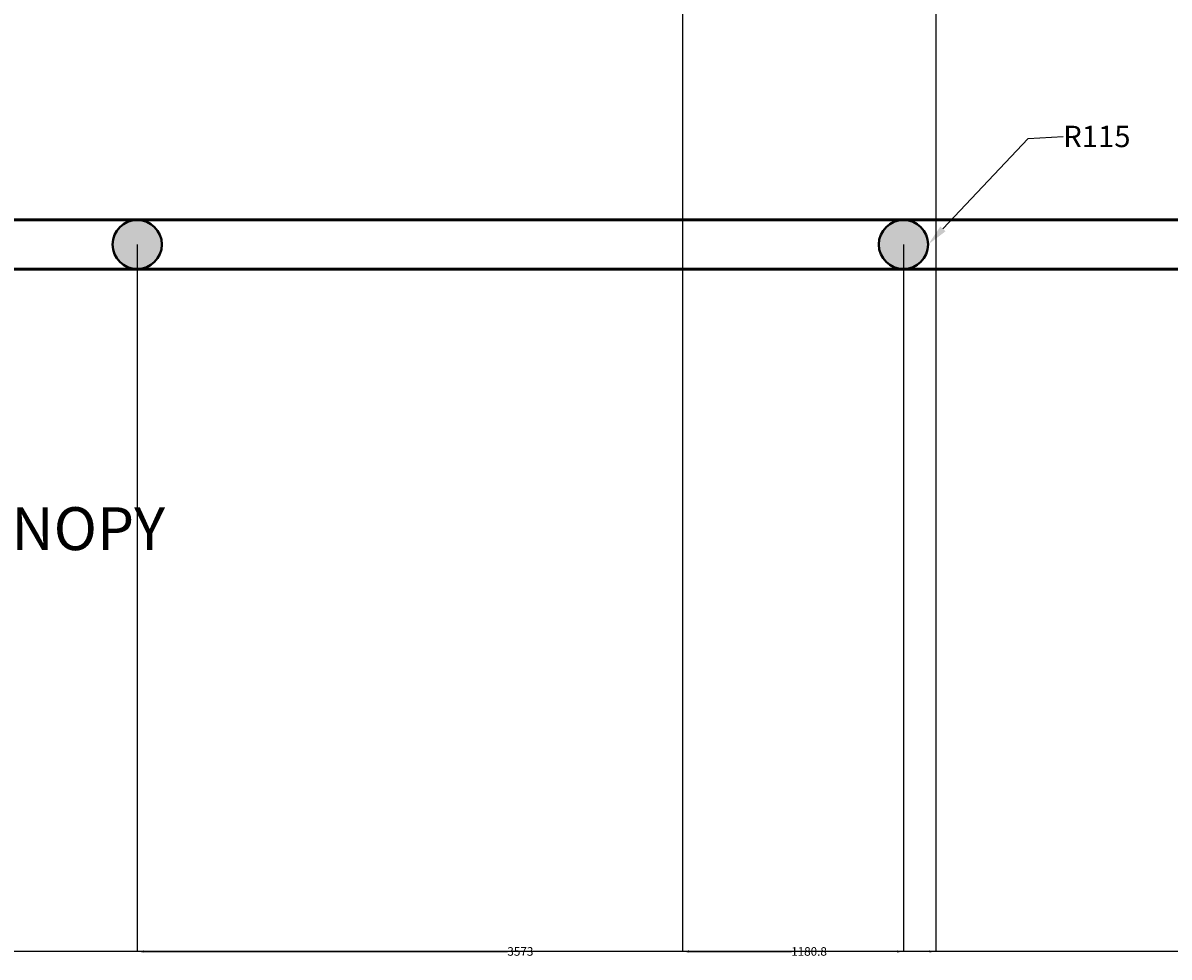
# Model space of a CAD drawing. Units: millimetres. Extents: x -17156 to 39375, y -45872 to -24892.
# Tile 5 of 12: x 7 to 5351, y -45872 to -41514. Entities that reach past the tile are written whole.
import ezdxf
from ezdxf import colors
from ezdxf.entities.mleader import LeaderData, LeaderLine
from ezdxf.math import Vec2, Vec3

# ---------------------------------------------------------------- set-up
doc = ezdxf.new("R2010")
doc.units = ezdxf.units.MM
doc.header["$MEASUREMENT"] = 0
for name, color, linetype, lineweight in [('A-ANNO-DIMS', 2, 'Continuous', 18), ('A-ANNO-TEXT', 4, 'Continuous', 18), ('A-COLS', 7, 'Continuous', 40), ('WALLS', 5, 'Continuous', 50)]:
    doc.layers.add(name, color=color, linetype=linetype, lineweight=lineweight)
doc.layers.add('A-COLS-PATT', color=114, linetype='Continuous', lineweight=13, true_color=0x139b48)
doc.styles.get("Standard").update_dxf_attribs({"font": 'arial.ttf'})
doc.dimstyles.get("Standard").update_dxf_attribs({"dimtxt": 40, "dimasz": 30.18, "dimexe": 0, "dimexo": 0.0625, "dimgap": 0.09, "dimtad": 0, "dimtih": 1, "dimtoh": 1, "dimdec": 0, "dimzin": 0, "dimdsep": 46, "dimtxsty": 'Standard', "dimcen": 0.09, "dimadec": 0, "dimazin": 0, "dimtfac": 1, "dimtdec": 0, "dimtofl": 0, "dimtmove": 0, "dimatfit": 3, "dimfxl": 1, "dimtolj": 1, "dimtzin": 0, "dimarcsym": 0})

# ---------------------------------------------------------------- blocks, each defined once
blk = doc.blocks.new('*D146')
at = {"layer": 'A-ANNO-DIMS', "color": 0, "lineweight": -2, "transparency": 16777216}
for p, q in [((-14867.3, -42732.9), (-14867.3, -45845.8)), ((13042.7, -42732.9), (13042.7, -45845.8)), ((-14837.2, -45845.8), (-988, -45845.8)), ((13012.5, -45845.8), (-836.7, -45845.8))]:
    blk.add_line(p, q, dxfattribs=at)
at = {"layer": 'A-ANNO-DIMS', "color": 0, "lineweight": 100, "transparency": 16777216}
for points in [[(-14837.2, -45840.8), (-14837.2, -45850.9), (-14867.3, -45845.8)], [(13012.5, -45840.8), (13012.5, -45850.9), (13042.7, -45845.8)]]:
    blk.add_solid(points, dxfattribs=at)
at = {"layer": 'Defpoints', "color": 0, "lineweight": 100, "transparency": 16777216}
for p in [(-14867.3, -42732.8), (13042.7, -42732.8), (13042.7, -45845.8)]:
    blk.add_point(p, dxfattribs=at)
at = {"layer": 'A-ANNO-DIMS', "color": 0, "transparency": 16777216, "insert": (-912.3, -45845.8), "char_height": 40, "attachment_point": 5}
blk.add_mtext('\\A1;27910', dxfattribs=at)
blk = doc.blocks.new('*D150')
at = {"layer": 'A-ANNO-DIMS', "color": 0, "lineweight": -2, "transparency": 16777216}
for p, q in [((3081.8, -35067.9), (3081.8, -45845.8)), ((4262.7, -35067.9), (4262.7, -45845.8)), ((3112, -45845.8), (3591, -45845.8)), ((4232.5, -45845.8), (3753.5, -45845.8))]:
    blk.add_line(p, q, dxfattribs=at)
at = {"layer": 'A-ANNO-DIMS', "color": 0, "lineweight": 100, "transparency": 16777216}
for points in [[(3112, -45840.8), (3112, -45850.9), (3081.8, -45845.8)], [(4232.5, -45840.8), (4232.5, -45850.9), (4262.7, -45845.8)]]:
    blk.add_solid(points, dxfattribs=at)
at = {"layer": 'Defpoints', "color": 0, "lineweight": 100, "transparency": 16777216}
for p in [(3081.8, -35067.8), (4262.7, -35067.8), (4262.7, -45845.8)]:
    blk.add_point(p, dxfattribs=at)
at = {"layer": 'A-ANNO-DIMS', "color": 0, "transparency": 16777216, "insert": (3672.2, -45845.8), "char_height": 40, "attachment_point": 5}
blk.add_mtext('\\A1;1180.8', dxfattribs=at)
blk = doc.blocks.new('*D153')
at = {"layer": 'A-ANNO-DIMS', "color": 0, "lineweight": -2, "transparency": 16777216}
for p, q in [((539.7, -42547.9), (539.7, -45845.8)), ((4112.7, -42547.9), (4112.7, -45845.8)), ((569.8, -45845.8), (2266.3, -45845.8)), ((4082.5, -45845.8), (2386, -45845.8))]:
    blk.add_line(p, q, dxfattribs=at)
at = {"layer": 'A-ANNO-DIMS', "color": 0, "lineweight": 100, "transparency": 16777216}
for points in [[(569.8, -45840.8), (569.8, -45850.9), (539.7, -45845.8)], [(4082.5, -45840.8), (4082.5, -45850.9), (4112.7, -45845.8)]]:
    blk.add_solid(points, dxfattribs=at)
at = {"layer": 'Defpoints', "color": 0, "lineweight": 100, "transparency": 16777216}
for p in [(539.7, -42547.8), (4112.7, -42547.8), (4112.7, -45845.8)]:
    blk.add_point(p, dxfattribs=at)
at = {"layer": 'A-ANNO-DIMS', "color": 0, "transparency": 16777216, "insert": (2326.2, -45845.8), "char_height": 40, "attachment_point": 5}
blk.add_mtext('\\A1;3573', dxfattribs=at)

msp = doc.modelspace()

# ---------------------------------------------------------------- hatches: boundary and pattern name
at = {"layer": 'A-COLS-PATT'}
h = msp.add_hatch(color=256, dxfattribs=at)
h.dxf.hatch_style = 1
h.paths.add_polyline_path([(-6007.35, -42547.85, 1), (-6237.35, -42547.85, 1)])
h.paths.add_polyline_path([(-2699.35, -42547.85, 1), (-2469.35, -42547.85, 1)])
h.paths.add_polyline_path([(424.65, -42547.85, 1), (654.65, -42547.85, 1)])
h.paths.add_polyline_path([(3997.65, -42547.85, 1), (4227.65, -42547.85, 1)])
h.paths.add_polyline_path([(1581.84, -34499.85), (1481.84, -34499.85), (1481.84, -34599.85), (1581.84, -34599.85)])
h.paths.add_polyline_path([(3181.84, -34499.85), (3081.84, -34499.85), (3081.84, -34599.85), (3181.84, -34599.85)])
h.paths.add_polyline_path([(-162.32, -34499.85), (-262.32, -34499.85), (-262.32, -34599.85), (-162.32, -34599.85)])
h.paths.add_polyline_path([(-1762.32, -34499.85), (-1862.32, -34499.85), (-1862.32, -34599.85), (-1762.32, -34599.85)])
h.paths.add_polyline_path([(-3445.85, -34499.85), (-3545.85, -34499.85), (-3545.85, -34599.85), (-3445.85, -34599.85)])
h.paths.add_polyline_path([(-5045.85, -34499.85), (-5145.85, -34499.85), (-5145.85, -34599.85), (-5045.85, -34599.85)])

# ---------------------------------------------------------------- linework, layer by layer
at = {"layer": 'A-COLS'}
for centre in [(539.65, -42547.85), (4112.65, -42547.85)]:
    msp.add_circle(centre, 115, dxfattribs=at)
at = {"layer": 'WALLS'}
for p, q in [((12592.65, -42432.85), (-10997.35, -42432.85)), ((12822.65, -42662.85), (-14797.35, -42662.85))]:
    msp.add_line(p, q, dxfattribs=at)

# ---------------------------------------------------------------- dimensions: what is measured, and where the dimension line sits
at = {"layer": 'A-ANNO-DIMS'}
for base, p1, p2, override, picture, middle in [((4262.65, -45845.85), (3081.84, -35067.85), (4262.65, -35067.85), {"dimdec": 1, "dimlfac": 1, "dimrnd": 0, "dimzin": 0, "dimdsep": 46, "dimlunit": 2}, '*D150', (3672.24, -45845.85)), ((4112.65, -45845.85), (539.65, -42547.85), (4112.65, -42547.85), {"dimdec": 0, "dimlfac": 1, "dimrnd": 0, "dimzin": 0, "dimdsep": 46, "dimlunit": 2}, '*D153', (2326.15, -45845.85)), ((13042.65, -45845.85), (-14867.35, -42732.85), (13042.65, -42732.85), {"dimdec": 0, "dimlfac": 1, "dimrnd": 0, "dimzin": 0, "dimdsep": 46, "dimlunit": 2}, '*D146', (-912.35, -45845.85))]:
    dim = msp.add_linear_dim(base=base, p1=p1, p2=p2, dimstyle='Standard', override=override, dxfattribs=at)
    dim.commit()
    dim.dimension.update_dxf_attribs({"geometry": picture, "text_midpoint": middle})

# ---------------------------------------------------------------- leaders
at = {"layer": 'A-ANNO-TEXT'}
ml = msp.add_multileader_mtext('Standard', dxfattribs=at)
ml.set_content('{\\C4;R115}', color=256)
ml.set_leader_properties()
ml.build(insert=Vec2(0, 0))
ml.multileader.update_dxf_attribs({"dogleg_length": 0.36, "arrow_head_size": 100})
ctx = ml.context
ctx.base_point, ctx.char_height, ctx.arrow_head_size, ctx.landing_gap_size, ctx.plane_origin = Vec3(4857.3, -42044.44), 100, 100, 0.09, Vec3(4227.65, -42547.85)
notes = []
notes.append((ctx, [(1, (1, 1, 0), (4856.94, -42044.44), (1, 0), 0.36, [(0, [(4227.65, -42547.85), (4694.69, -42053.97)], 0, [])])]))
ctx.mtext.insert, ctx.mtext.flow_direction = Vec3(4857.39, -41993.58), 5
ml = msp.add_multileader_mtext('Standard', dxfattribs=at)
ml.set_content('{\\C4;CANOPY}', color=256)
ml.set_leader_properties()
ml.build(insert=Vec2(0, 0))
ml.multileader.update_dxf_attribs({"dogleg_length": 0.36, "arrow_head_size": 200})
ctx = ml.context
ctx.base_point, ctx.char_height, ctx.arrow_head_size, ctx.landing_gap_size, ctx.plane_origin = Vec3(-387.3, -43875.13), 200, 200, 0.09, Vec3(-1022.35, -43875.13)
notes.append((ctx, [(0, (1, 1, 0), (-387.66, -43875.13), (1, 0), 0.36, [(0, [(-1022.35, -43875.13)], 0, [])])]))
ctx.mtext.insert, ctx.mtext.flow_direction = Vec3(-387.21, -43773.42), 5
for ctx, leaders in notes:
    for number, flags, end, landing, length, lines in leaders:
        leader = LeaderData()
        leader.index, (leader.has_last_leader_line, leader.has_dogleg_vector, leader.attachment_direction) = number, flags
        leader.last_leader_point, leader.dogleg_vector, leader.dogleg_length = Vec3(end), Vec3(landing), length
        for number, points, colour, breaks in lines:
            line = LeaderLine()
            line.index, line.vertices, line.color, line.breaks = number, Vec3.list(points), colors.encode_raw_color(colour), breaks
            leader.lines.append(line)
        ctx.leaders.append(leader)

doc.saveas('drawing.dxf')
